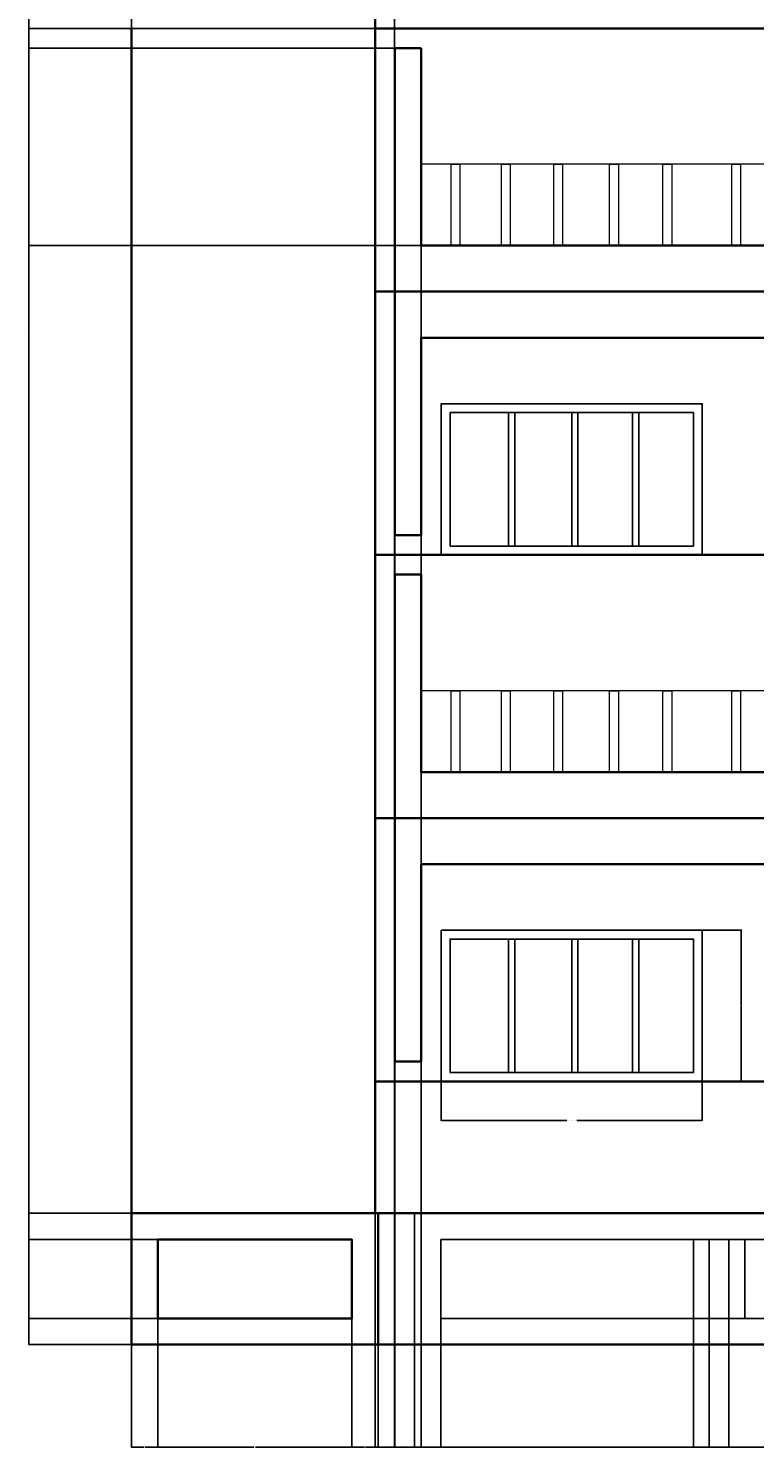
# Model space of a CAD drawing. Units: inches. Extents: x -26 to 668, y -42 to 976.
# Tile 1 of 3: x -26 to 305, y -42 to 605. Entities that reach past the tile are written whole.
import ezdxf

# ---------------------------------------------------------------- set-up
doc = ezdxf.new("R2010")
doc.units = ezdxf.units.IN
doc.header["$MEASUREMENT"] = 0
for name, color, linetype, lineweight in [('A-ANNO-DIMS', 2, 'Continuous', 18), ('A-DOOR', 3, 'Continuous', 25), ('A-ELEV', 7, 'Continuous', 35), ('A-FLOR-HRAL', 8, 'Continuous', 18), ('A-GLAZ', 4, 'Continuous', 25)]:
    doc.layers.add(name, color=color, linetype=linetype, lineweight=lineweight)
doc.styles.get("Standard").update_dxf_attribs({"font": 'arial.ttf'})
doc.dimstyles.get("Standard").update_dxf_attribs({"dimtxt": 0.18, "dimasz": 0.18, "dimexe": 0.18, "dimexo": 0.0625, "dimgap": 0.09, "dimtad": 0, "dimtih": 1, "dimtoh": 1, "dimdec": 4, "dimzin": 0, "dimdsep": 46, "dimtxsty": 'Standard', "dimcen": 0.09, "dimadec": 0, "dimazin": 0, "dimtfac": 1, "dimtdec": 4, "dimtofl": 0, "dimtmove": 0, "dimatfit": 3, "dimfxl": 1, "dimtolj": 1, "dimtzin": 0, "dimarcsym": 0})

# ---------------------------------------------------------------- blocks, each defined once
blk = doc.blocks.new('WIN-SLIDING-4P')
for p, q in [((192.66, 189.86), (192.66, 128.96)), ((195.46, 189.86), (195.46, 128.96)), ((221.46, 189.86), (221.46, 128.96)), ((224.25, 189.86), (224.25, 128.96)), ((249.2, 189.86), (249.2, 128.96)), ((251.99, 189.86), (251.99, 128.96))]:
    blk.add_line(p, q)
for points in [[(162.01, 124.96), (280.91, 124.96), (280.91, 193.86), (162.01, 193.86)], [(166.01, 128.96), (276.91, 128.96), (276.91, 189.86), (166.01, 189.86)]]:
    blk.add_lwpolyline(points, close=True)
blk = doc.blocks.new('RAILING-BALCONY')
for points in [[(331.17, 145.96), (599.79, 145.96), (599.79, 183.06), (331.17, 183.06)], [(344.86, 183.06), (348.85, 183.06), (348.85, 145.96), (344.86, 145.96)], [(367.74, 183.06), (371.72, 183.06), (371.72, 145.96), (367.74, 145.96)], [(391.66, 183.06), (395.64, 183.06), (395.64, 145.96), (391.66, 145.96)], [(417.04, 183.06), (421.03, 183.06), (421.03, 145.96), (417.04, 145.96)], [(441.38, 183.06), (445.37, 183.06), (445.37, 145.96), (441.38, 145.96)], [(472.69, 183.06), (476.68, 183.06), (476.68, 145.96), (472.69, 145.96)], [(501.02, 183.06), (505, 183.06), (505, 145.96), (501.02, 145.96)], [(530.39, 183.06), (534.38, 183.06), (534.38, 145.96), (530.39, 145.96)], [(556.62, 183.06), (560.61, 183.06), (560.61, 145.96), (556.62, 145.96)], [(580.54, 183.06), (584.53, 183.06), (584.53, 145.96), (580.54, 145.96)]]:
    blk.add_lwpolyline(points, close=True)
blk = doc.blocks.new('*D5')
at = {"layer": 'A-ANNO-DIMS', "color": 0, "lineweight": -2, "transparency": 16777216}
for p, q in [((162.01, 124.9), (162.01, 106.95)), ((280.91, 124.9), (280.91, 106.95)), ((162.19, 107.13), (219.17, 107.13)), ((280.73, 107.13), (223.74, 107.13))]:
    blk.add_line(p, q, dxfattribs=at)
at = {"layer": 'A-ANNO-DIMS', "color": 0, "transparency": 16777216}
for points in [[(162.19, 107.16), (162.19, 107.1), (162.01, 107.13)], [(280.73, 107.16), (280.73, 107.1), (280.91, 107.13)]]:
    blk.add_solid(points, dxfattribs=at)
at = {"layer": 'Defpoints', "color": 0, "transparency": 16777216}
for p in [(162.01, 124.96), (280.91, 124.96), (280.91, 107.13)]:
    blk.add_point(p, dxfattribs=at)
at = {"layer": 'A-ANNO-DIMS', "color": 0, "transparency": 16777216, "insert": (221.46, 107.13), "char_height": 0.18, "attachment_point": 5}
blk.add_mtext('\\A1;4-PANEL SLIDING WINDOW 119 TYP.', dxfattribs=at)
blk = doc.blocks.new('*D6')
at = {"layer": 'A-ANNO-DIMS', "color": 0, "lineweight": -2, "transparency": 16777216}
for p, q in [((280.97, 193.86), (298.92, 193.86)), ((298.74, 193.68), (298.74, 159.59)), ((298.74, 125.14), (298.74, 159.23)), ((280.97, 124.96), (298.92, 124.96))]:
    blk.add_line(p, q, dxfattribs=at)
at = {"layer": 'A-ANNO-DIMS', "color": 0, "transparency": 16777216}
for points in [[(298.71, 193.68), (298.77, 193.68), (298.74, 193.86)], [(298.71, 125.14), (298.77, 125.14), (298.74, 124.96)]]:
    blk.add_solid(points, dxfattribs=at)
at = {"layer": 'Defpoints', "color": 0, "transparency": 16777216}
for p in [(280.91, 193.86), (298.74, 193.86), (280.91, 124.96)]:
    blk.add_point(p, dxfattribs=at)
at = {"layer": 'A-ANNO-DIMS', "color": 0, "transparency": 16777216, "insert": (298.74, 159.41), "char_height": 0.18, "attachment_point": 5}
blk.add_mtext('\\A1;69 TYP.', dxfattribs=at)
blk = doc.blocks.new('*D8')
at = {"layer": 'A-ANNO-DIMS', "color": 0, "lineweight": -2, "transparency": 16777216}
for p, q in [((140.59, 928.96), (-26.14, 928.96)), ((-25.96, 928.78), (-25.96, 467.14)), ((-25.96, 5.14), (-25.96, 466.78)), ((20.73, 4.96), (-26.14, 4.96))]:
    blk.add_line(p, q, dxfattribs=at)
at = {"layer": 'A-ANNO-DIMS', "color": 0, "transparency": 16777216}
for points in [[(-25.99, 928.78), (-25.93, 928.78), (-25.96, 928.96)], [(-25.99, 5.14), (-25.93, 5.14), (-25.96, 4.96)]]:
    blk.add_solid(points, dxfattribs=at)
at = {"layer": 'Defpoints', "color": 0, "transparency": 16777216}
for p in [(-25.96, 928.96), (140.65, 928.96), (20.79, 4.96)]:
    blk.add_point(p, dxfattribs=at)
at = {"layer": 'A-ANNO-DIMS', "color": 0, "transparency": 16777216, "insert": (-25.96, 466.96), "char_height": 0.18, "attachment_point": 5}
blk.add_mtext('\\A1;924', dxfattribs=at)
blk = doc.blocks.new('*D22')
at = {"layer": 'A-ANNO-DIMS', "color": 0, "lineweight": -2, "transparency": 16777216}
for p, q in [((140.65, 844.9), (140.65, -41.97)), ((483.43, 844.9), (483.43, -41.97)), ((140.83, -41.79), (311.65, -41.79)), ((483.25, -41.79), (312.43, -41.79))]:
    blk.add_line(p, q, dxfattribs=at)
at = {"layer": 'A-ANNO-DIMS', "color": 0, "transparency": 16777216}
for points in [[(140.83, -41.76), (140.83, -41.82), (140.65, -41.79)], [(483.25, -41.76), (483.25, -41.82), (483.43, -41.79)]]:
    blk.add_solid(points, dxfattribs=at)
at = {"layer": 'Defpoints', "color": 0, "transparency": 16777216}
for p in [(140.65, 844.96), (483.43, 844.96), (483.43, -41.79)]:
    blk.add_point(p, dxfattribs=at)
at = {"layer": 'A-ANNO-DIMS', "color": 0, "transparency": 16777216, "insert": (312.04, -41.79), "char_height": 0.18, "attachment_point": 5}
blk.add_mtext('\\A1;342.8', dxfattribs=at)
blk = doc.blocks.new('*D28')
at = {"layer": 'A-ANNO-DIMS', "color": 0, "lineweight": -2, "transparency": 16777216}
for p, q in [((131.83, 604.9), (131.83, -41.97)), ((140.83, 595.9), (140.83, -41.97)), ((132.01, -41.79), (136.19, -41.79)), ((140.65, -41.79), (136.48, -41.79))]:
    blk.add_line(p, q, dxfattribs=at)
at = {"layer": 'A-ANNO-DIMS', "color": 0, "transparency": 16777216}
for points in [[(132.01, -41.76), (132.01, -41.82), (131.83, -41.79)], [(140.65, -41.76), (140.65, -41.82), (140.83, -41.79)]]:
    blk.add_solid(points, dxfattribs=at)
at = {"layer": 'Defpoints', "color": 0, "transparency": 16777216}
for p in [(131.83, 604.96), (140.83, 595.96), (140.83, -41.79)]:
    blk.add_point(p, dxfattribs=at)
at = {"layer": 'A-ANNO-DIMS', "color": 0, "transparency": 16777216, "insert": (136.33, -41.79), "char_height": 0.18, "attachment_point": 5}
blk.add_mtext('\\A1;9', dxfattribs=at)
blk = doc.blocks.new('*D29')
at = {"layer": 'A-ANNO-DIMS', "color": 0, "lineweight": -2, "transparency": 16777216}
for p, q in [((140.83, 595.9), (140.83, -41.97)), ((152.83, 505.9), (152.83, -41.97)), ((141.01, -41.79), (146.63, -41.79)), ((152.65, -41.79), (147.04, -41.79))]:
    blk.add_line(p, q, dxfattribs=at)
at = {"layer": 'A-ANNO-DIMS', "color": 0, "transparency": 16777216}
for points in [[(141.01, -41.76), (141.01, -41.82), (140.83, -41.79)], [(152.65, -41.76), (152.65, -41.82), (152.83, -41.79)]]:
    blk.add_solid(points, dxfattribs=at)
at = {"layer": 'Defpoints', "color": 0, "transparency": 16777216}
for p in [(140.83, 595.96), (152.83, 505.96), (152.83, -41.79)]:
    blk.add_point(p, dxfattribs=at)
at = {"layer": 'A-ANNO-DIMS', "color": 0, "transparency": 16777216, "insert": (146.83, -41.79), "char_height": 0.18, "attachment_point": 5}
blk.add_mtext('\\A1;12', dxfattribs=at)
blk = doc.blocks.new('*D30')
at = {"layer": 'A-ANNO-DIMS', "color": 0, "lineweight": -2, "transparency": 16777216}
for p, q in [((152.83, 505.9), (152.83, -41.97)), ((310.17, 505.9), (310.17, -41.97)), ((153.01, -41.79), (231.05, -41.79)), ((309.99, -41.79), (231.96, -41.79))]:
    blk.add_line(p, q, dxfattribs=at)
at = {"layer": 'A-ANNO-DIMS', "color": 0, "transparency": 16777216}
for points in [[(153.01, -41.76), (153.01, -41.82), (152.83, -41.79)], [(309.99, -41.76), (309.99, -41.82), (310.17, -41.79)]]:
    blk.add_solid(points, dxfattribs=at)
at = {"layer": 'Defpoints', "color": 0, "transparency": 16777216}
for p in [(152.83, 505.96), (310.17, 505.96), (310.17, -41.79)]:
    blk.add_point(p, dxfattribs=at)
at = {"layer": 'A-ANNO-DIMS', "color": 0, "transparency": 16777216, "insert": (231.5, -41.79), "char_height": 0.18, "attachment_point": 5}
blk.add_mtext('\\A1;157.34', dxfattribs=at)
blk = doc.blocks.new('*D38')
at = {"layer": 'A-ANNO-DIMS', "color": 0, "lineweight": -2, "transparency": 16777216}
for p, q in [((140.77, 595.96), (-26.14, 595.96)), ((-25.96, 595.78), (-25.96, 551.14)), ((-25.96, 506.14), (-25.96, 550.78)), ((152.77, 505.96), (-26.14, 505.96))]:
    blk.add_line(p, q, dxfattribs=at)
at = {"layer": 'A-ANNO-DIMS', "color": 0, "transparency": 16777216}
for points in [[(-25.99, 595.78), (-25.93, 595.78), (-25.96, 595.96)], [(-25.99, 506.14), (-25.93, 506.14), (-25.96, 505.96)]]:
    blk.add_solid(points, dxfattribs=at)
at = {"layer": 'Defpoints', "color": 0, "transparency": 16777216}
for p in [(-25.96, 595.96), (140.83, 595.96), (152.83, 505.96)]:
    blk.add_point(p, dxfattribs=at)
at = {"layer": 'A-ANNO-DIMS', "color": 0, "transparency": 16777216, "insert": (-25.96, 550.96), "char_height": 0.18, "attachment_point": 5}
blk.add_mtext('\\A1;90', dxfattribs=at)
blk = doc.blocks.new('*D39')
at = {"layer": 'A-ANNO-DIMS', "color": 0, "lineweight": -2, "transparency": 16777216}
for p, q in [((131.77, 604.96), (-26.14, 604.96)), ((-25.96, 604.78), (-25.96, 600.64)), ((140.77, 595.96), (-26.14, 595.96)), ((-25.96, 596.14), (-25.96, 600.28))]:
    blk.add_line(p, q, dxfattribs=at)
at = {"layer": 'A-ANNO-DIMS', "color": 0, "transparency": 16777216}
for points in [[(-25.99, 604.78), (-25.93, 604.78), (-25.96, 604.96)], [(-25.99, 596.14), (-25.93, 596.14), (-25.96, 595.96)]]:
    blk.add_solid(points, dxfattribs=at)
at = {"layer": 'Defpoints', "color": 0, "transparency": 16777216}
for p in [(-25.96, 604.96), (131.83, 604.96), (140.83, 595.96)]:
    blk.add_point(p, dxfattribs=at)
at = {"layer": 'A-ANNO-DIMS', "color": 0, "transparency": 16777216, "insert": (-25.96, 600.46), "char_height": 0.18, "attachment_point": 5}
blk.add_mtext('\\A1;9', dxfattribs=at)
blk = doc.blocks.new('*D40')
at = {"layer": 'A-ANNO-DIMS', "color": 0, "lineweight": -2, "transparency": 16777216}
for p, q in [((140.77, 613.96), (-26.14, 613.96)), ((-25.96, 613.78), (-25.96, 609.64)), ((-25.96, 605.14), (-25.96, 609.28)), ((131.77, 604.96), (-26.14, 604.96))]:
    blk.add_line(p, q, dxfattribs=at)
at = {"layer": 'A-ANNO-DIMS', "color": 0, "transparency": 16777216}
for points in [[(-25.99, 613.78), (-25.93, 613.78), (-25.96, 613.96)], [(-25.99, 605.14), (-25.93, 605.14), (-25.96, 604.96)]]:
    blk.add_solid(points, dxfattribs=at)
at = {"layer": 'Defpoints', "color": 0, "transparency": 16777216}
for p in [(-25.96, 613.96), (140.83, 613.96), (131.83, 604.96)]:
    blk.add_point(p, dxfattribs=at)
at = {"layer": 'A-ANNO-DIMS', "color": 0, "transparency": 16777216, "insert": (-25.96, 609.46), "char_height": 0.18, "attachment_point": 5}
blk.add_mtext('\\A1;9', dxfattribs=at)
blk = doc.blocks.new('*D47')
at = {"layer": 'A-ANNO-DIMS', "color": 0, "lineweight": -2, "transparency": 16777216}
for p, q in [((32.79, 16.9), (32.79, -41.97)), ((20.79, 4.9), (20.79, -41.97)), ((20.97, -41.79), (26.58, -41.79)), ((32.61, -41.79), (27, -41.79))]:
    blk.add_line(p, q, dxfattribs=at)
at = {"layer": 'A-ANNO-DIMS', "color": 0, "transparency": 16777216}
for points in [[(20.97, -41.76), (20.97, -41.82), (20.79, -41.79)], [(32.61, -41.76), (32.61, -41.82), (32.79, -41.79)]]:
    blk.add_solid(points, dxfattribs=at)
at = {"layer": 'Defpoints', "color": 0, "transparency": 16777216}
for p in [(32.79, 16.96), (20.79, 4.96), (32.79, -41.79)]:
    blk.add_point(p, dxfattribs=at)
at = {"layer": 'A-ANNO-DIMS', "color": 0, "transparency": 16777216, "insert": (26.79, -41.79), "char_height": 0.18, "attachment_point": 5}
blk.add_mtext('\\A1;12', dxfattribs=at)
blk = doc.blocks.new('*D48')
at = {"layer": 'A-ANNO-DIMS', "color": 0, "lineweight": -2, "transparency": 16777216}
for p, q in [((32.79, 16.9), (32.79, -41.97)), ((121.22, 16.9), (121.22, -41.97)), ((32.97, -41.79), (76.61, -41.79)), ((121.04, -41.79), (77.4, -41.79))]:
    blk.add_line(p, q, dxfattribs=at)
at = {"layer": 'A-ANNO-DIMS', "color": 0, "transparency": 16777216}
for points in [[(32.97, -41.76), (32.97, -41.82), (32.79, -41.79)], [(121.04, -41.76), (121.04, -41.82), (121.22, -41.79)]]:
    blk.add_solid(points, dxfattribs=at)
at = {"layer": 'Defpoints', "color": 0, "transparency": 16777216}
for p in [(32.79, 16.96), (121.22, 16.96), (121.22, -41.79)]:
    blk.add_point(p, dxfattribs=at)
at = {"layer": 'A-ANNO-DIMS', "color": 0, "transparency": 16777216, "insert": (77.01, -41.79), "char_height": 0.18, "attachment_point": 5}
blk.add_mtext('\\A1;88.43', dxfattribs=at)
blk = doc.blocks.new('*D49')
at = {"layer": 'A-ANNO-DIMS', "color": 0, "lineweight": -2, "transparency": 16777216}
for p, q in [((121.22, 16.9), (121.22, -41.97)), ((133.22, 4.9), (133.22, -41.97)), ((121.4, -41.79), (127.01, -41.79)), ((133.04, -41.79), (127.43, -41.79))]:
    blk.add_line(p, q, dxfattribs=at)
at = {"layer": 'A-ANNO-DIMS', "color": 0, "transparency": 16777216}
for points in [[(121.4, -41.76), (121.4, -41.82), (121.22, -41.79)], [(133.04, -41.76), (133.04, -41.82), (133.22, -41.79)]]:
    blk.add_solid(points, dxfattribs=at)
at = {"layer": 'Defpoints', "color": 0, "transparency": 16777216}
for p in [(121.22, 16.96), (133.22, 4.96), (133.22, -41.79)]:
    blk.add_point(p, dxfattribs=at)
at = {"layer": 'A-ANNO-DIMS', "color": 0, "transparency": 16777216, "insert": (127.22, -41.79), "char_height": 0.18, "attachment_point": 5}
blk.add_mtext('\\A1;12', dxfattribs=at)
blk = doc.blocks.new('*D50')
at = {"layer": 'A-ANNO-DIMS', "color": 0, "lineweight": -2, "transparency": 16777216}
for p, q in [((133.22, 4.9), (133.22, -41.97)), ((149.75, 4.9), (149.75, -41.97)), ((133.4, -41.79), (141.03, -41.79)), ((149.57, -41.79), (141.94, -41.79))]:
    blk.add_line(p, q, dxfattribs=at)
at = {"layer": 'A-ANNO-DIMS', "color": 0, "transparency": 16777216}
for points in [[(133.4, -41.76), (133.4, -41.82), (133.22, -41.79)], [(149.57, -41.76), (149.57, -41.82), (149.75, -41.79)]]:
    blk.add_solid(points, dxfattribs=at)
at = {"layer": 'Defpoints', "color": 0, "transparency": 16777216}
for p in [(133.22, 4.96), (149.75, 4.96), (149.75, -41.79)]:
    blk.add_point(p, dxfattribs=at)
at = {"layer": 'A-ANNO-DIMS', "color": 0, "transparency": 16777216, "insert": (141.49, -41.79), "char_height": 0.18, "attachment_point": 5}
blk.add_mtext('\\A1;16.527', dxfattribs=at)
blk = doc.blocks.new('*D51')
at = {"layer": 'A-ANNO-DIMS', "color": 0, "lineweight": -2, "transparency": 16777216}
for p, q in [((161.75, 16.9), (161.75, -41.97)), ((149.75, 4.9), (149.75, -41.97)), ((149.93, -41.79), (155.54, -41.79)), ((161.57, -41.79), (155.96, -41.79))]:
    blk.add_line(p, q, dxfattribs=at)
at = {"layer": 'A-ANNO-DIMS', "color": 0, "transparency": 16777216}
for points in [[(149.93, -41.76), (149.93, -41.82), (149.75, -41.79)], [(161.57, -41.76), (161.57, -41.82), (161.75, -41.79)]]:
    blk.add_solid(points, dxfattribs=at)
at = {"layer": 'Defpoints', "color": 0, "transparency": 16777216}
for p in [(161.75, 16.96), (149.75, 4.96), (161.75, -41.79)]:
    blk.add_point(p, dxfattribs=at)
at = {"layer": 'A-ANNO-DIMS', "color": 0, "transparency": 16777216, "insert": (155.75, -41.79), "char_height": 0.18, "attachment_point": 5}
blk.add_mtext('\\A1;12', dxfattribs=at)
blk = doc.blocks.new('*D52')
at = {"layer": 'A-ANNO-DIMS', "color": 0, "lineweight": -2, "transparency": 16777216}
for p, q in [((161.75, 16.9), (161.75, -41.97)), ((276.93, 16.9), (276.93, -41.97)), ((161.93, -41.79), (218.89, -41.79)), ((276.75, -41.79), (219.8, -41.79))]:
    blk.add_line(p, q, dxfattribs=at)
at = {"layer": 'A-ANNO-DIMS', "color": 0, "transparency": 16777216}
for points in [[(161.93, -41.76), (161.93, -41.82), (161.75, -41.79)], [(276.75, -41.76), (276.75, -41.82), (276.93, -41.79)]]:
    blk.add_solid(points, dxfattribs=at)
at = {"layer": 'Defpoints', "color": 0, "transparency": 16777216}
for p in [(161.75, 16.96), (276.93, 16.96), (276.93, -41.79)]:
    blk.add_point(p, dxfattribs=at)
at = {"layer": 'A-ANNO-DIMS', "color": 0, "transparency": 16777216, "insert": (219.34, -41.79), "char_height": 0.18, "attachment_point": 5}
blk.add_mtext('\\A1;115.18', dxfattribs=at)
blk = doc.blocks.new('*D53')
at = {"layer": 'A-ANNO-DIMS', "color": 0, "lineweight": -2, "transparency": 16777216}
for p, q in [((276.93, 16.9), (276.93, -41.97)), ((284.11, 16.9), (284.11, -41.97)), ((277.11, -41.79), (280.13, -41.79)), ((283.93, -41.79), (280.91, -41.79))]:
    blk.add_line(p, q, dxfattribs=at)
at = {"layer": 'A-ANNO-DIMS', "color": 0, "transparency": 16777216}
for points in [[(277.11, -41.76), (277.11, -41.82), (276.93, -41.79)], [(283.93, -41.76), (283.93, -41.82), (284.11, -41.79)]]:
    blk.add_solid(points, dxfattribs=at)
at = {"layer": 'Defpoints', "color": 0, "transparency": 16777216}
for p in [(276.93, 16.96), (284.11, 16.96), (284.11, -41.79)]:
    blk.add_point(p, dxfattribs=at)
at = {"layer": 'A-ANNO-DIMS', "color": 0, "transparency": 16777216, "insert": (280.52, -41.79), "char_height": 0.18, "attachment_point": 5}
blk.add_mtext('\\A1;7.177', dxfattribs=at)
blk = doc.blocks.new('*D54')
at = {"layer": 'A-ANNO-DIMS', "color": 0, "lineweight": -2, "transparency": 16777216}
for p, q in [((284.11, 16.9), (284.11, -41.97)), ((293.12, 16.9), (293.12, -41.97)), ((284.29, -41.79), (288.22, -41.79)), ((292.94, -41.79), (289.01, -41.79))]:
    blk.add_line(p, q, dxfattribs=at)
at = {"layer": 'A-ANNO-DIMS', "color": 0, "transparency": 16777216}
for points in [[(284.29, -41.76), (284.29, -41.82), (284.11, -41.79)], [(292.94, -41.76), (292.94, -41.82), (293.12, -41.79)]]:
    blk.add_solid(points, dxfattribs=at)
at = {"layer": 'Defpoints', "color": 0, "transparency": 16777216}
for p in [(284.11, 16.96), (293.12, 16.96), (293.12, -41.79)]:
    blk.add_point(p, dxfattribs=at)
at = {"layer": 'A-ANNO-DIMS', "color": 0, "transparency": 16777216, "insert": (288.61, -41.79), "char_height": 0.18, "attachment_point": 5}
blk.add_mtext('\\A1;9.007', dxfattribs=at)
blk = doc.blocks.new('*D55')
at = {"layer": 'A-ANNO-DIMS', "color": 0, "lineweight": -2, "transparency": 16777216}
for p, q in [((293.12, 16.9), (293.12, -41.97)), ((381.21, 16.9), (381.21, -41.97)), ((293.3, -41.79), (336.86, -41.79)), ((381.03, -41.79), (337.47, -41.79))]:
    blk.add_line(p, q, dxfattribs=at)
at = {"layer": 'A-ANNO-DIMS', "color": 0, "transparency": 16777216}
for points in [[(293.3, -41.76), (293.3, -41.82), (293.12, -41.79)], [(381.03, -41.76), (381.03, -41.82), (381.21, -41.79)]]:
    blk.add_solid(points, dxfattribs=at)
at = {"layer": 'Defpoints', "color": 0, "transparency": 16777216}
for p in [(293.12, 16.96), (381.21, 16.96), (381.21, -41.79)]:
    blk.add_point(p, dxfattribs=at)
at = {"layer": 'A-ANNO-DIMS', "color": 0, "transparency": 16777216, "insert": (337.16, -41.79), "char_height": 0.18, "attachment_point": 5}
blk.add_mtext('\\A1;88.1', dxfattribs=at)
blk = doc.blocks.new('*D59')
at = {"layer": 'A-ANNO-DIMS', "color": 0, "lineweight": -2, "transparency": 16777216}
for p, q in [((32.73, 16.96), (-26.14, 16.96)), ((-25.96, 16.78), (-25.96, 11.14)), ((-25.96, 5.14), (-25.96, 10.78)), ((20.73, 4.96), (-26.14, 4.96))]:
    blk.add_line(p, q, dxfattribs=at)
at = {"layer": 'A-ANNO-DIMS', "color": 0, "transparency": 16777216}
for points in [[(-25.99, 16.78), (-25.93, 16.78), (-25.96, 16.96)], [(-25.99, 5.14), (-25.93, 5.14), (-25.96, 4.96)]]:
    blk.add_solid(points, dxfattribs=at)
at = {"layer": 'Defpoints', "color": 0, "transparency": 16777216}
for p in [(-25.96, 16.96), (32.79, 16.96), (20.79, 4.96)]:
    blk.add_point(p, dxfattribs=at)
at = {"layer": 'A-ANNO-DIMS', "color": 0, "transparency": 16777216, "insert": (-25.96, 10.96), "char_height": 0.18, "attachment_point": 5}
blk.add_mtext('\\A1;12', dxfattribs=at)
blk = doc.blocks.new('*D60')
at = {"layer": 'A-ANNO-DIMS', "color": 0, "lineweight": -2, "transparency": 16777216}
for p, q in [((32.73, 52.96), (-26.14, 52.96)), ((-25.96, 52.78), (-25.96, 35.14)), ((-25.96, 17.14), (-25.96, 34.78)), ((32.73, 16.96), (-26.14, 16.96))]:
    blk.add_line(p, q, dxfattribs=at)
at = {"layer": 'A-ANNO-DIMS', "color": 0, "transparency": 16777216}
for points in [[(-25.99, 52.78), (-25.93, 52.78), (-25.96, 52.96)], [(-25.99, 17.14), (-25.93, 17.14), (-25.96, 16.96)]]:
    blk.add_solid(points, dxfattribs=at)
at = {"layer": 'Defpoints', "color": 0, "transparency": 16777216}
for p in [(-25.96, 52.96), (32.79, 52.96), (32.79, 16.96)]:
    blk.add_point(p, dxfattribs=at)
at = {"layer": 'A-ANNO-DIMS', "color": 0, "transparency": 16777216, "insert": (-25.96, 34.96), "char_height": 0.18, "attachment_point": 5}
blk.add_mtext('\\A1;36', dxfattribs=at)
blk = doc.blocks.new('*D61')
at = {"layer": 'A-ANNO-DIMS', "color": 0, "lineweight": -2, "transparency": 16777216}
for p, q in [((20.73, 64.96), (-26.14, 64.96)), ((-25.96, 64.78), (-25.96, 59.14)), ((-25.96, 53.14), (-25.96, 58.78)), ((32.73, 52.96), (-26.14, 52.96))]:
    blk.add_line(p, q, dxfattribs=at)
at = {"layer": 'A-ANNO-DIMS', "color": 0, "transparency": 16777216}
for points in [[(-25.99, 64.78), (-25.93, 64.78), (-25.96, 64.96)], [(-25.99, 53.14), (-25.93, 53.14), (-25.96, 52.96)]]:
    blk.add_solid(points, dxfattribs=at)
at = {"layer": 'Defpoints', "color": 0, "transparency": 16777216}
for p in [(-25.96, 64.96), (20.79, 64.96), (32.79, 52.96)]:
    blk.add_point(p, dxfattribs=at)
at = {"layer": 'A-ANNO-DIMS', "color": 0, "transparency": 16777216, "insert": (-25.96, 58.96), "char_height": 0.18, "attachment_point": 5}
blk.add_mtext('\\A1;12', dxfattribs=at)
blk = doc.blocks.new('*D65')
at = {"layer": 'A-ANNO-DIMS', "color": 0, "lineweight": -2, "transparency": 16777216}
for p, q in [((20.79, 65.02), (20.79, 975.89)), ((20.97, 975.71), (75.86, 975.71)), ((131.65, 975.71), (76.77, 975.71)), ((131.83, 65.02), (131.83, 975.89))]:
    blk.add_line(p, q, dxfattribs=at)
at = {"layer": 'A-ANNO-DIMS', "color": 0, "transparency": 16777216}
for points in [[(20.97, 975.74), (20.97, 975.68), (20.79, 975.71)], [(131.65, 975.74), (131.65, 975.68), (131.83, 975.71)]]:
    blk.add_solid(points, dxfattribs=at)
at = {"layer": 'Defpoints', "color": 0, "transparency": 16777216}
for p in [(131.83, 975.71), (20.79, 64.96), (131.83, 64.96)]:
    blk.add_point(p, dxfattribs=at)
at = {"layer": 'A-ANNO-DIMS', "color": 0, "transparency": 16777216, "insert": (76.31, 975.71), "char_height": 0.18, "attachment_point": 5}
blk.add_mtext('\\A1;111.04', dxfattribs=at)

msp = doc.modelspace()

# ---------------------------------------------------------------- linework, layer by layer
at = {"layer": 'A-DOOR'}
for points in [[(149.7506, 64.9609), (402.2206, 64.9609), (402.2206, 4.9609), (149.7506, 4.9609)], [(161.7506, 52.9609), (390.2206, 52.9609), (390.2206, 16.9609), (161.7506, 16.9609)], [(284.1079, 16.9609), (276.9308, 16.9609), (276.9308, 52.9609), (284.1079, 52.9609)], [(300.2922, 16.9609), (293.1151, 16.9609), (293.1151, 52.9609), (300.2922, 52.9609)]]:
    msp.add_lwpolyline(points, close=True, dxfattribs=at)
at = {"layer": 'A-ELEV'}
for p, q in [((131.8349, 844.9609), (131.8349, 64.9609)), ((140.8349, 484.9609), (140.8349, 595.9609)), ((140.8349, 595.9609), (152.8349, 595.9609)), ((140.8349, 244.9609), (140.8349, 355.9609)), ((140.8349, 355.9609), (152.8349, 355.9609)), ((140.8349, 244.9609), (140.8349, 133.9609)), ((140.8349, 133.9609), (152.8349, 133.9609)), ((20.7944, 124.9609), (20.7944, 4.9609)), ((620.7944, 124.9609), (131.8349, 124.9609)), ((20.7944, 64.9609), (620.7944, 64.9609)), ((20.7944, 4.9609), (620.7944, 4.9609))]:
    msp.add_line(p, q, dxfattribs=at)
for points in [[(20.7944, 604.9609), (20.7944, 484.9609)], [(131.8349, 484.9609), (620.7944, 484.9609), (620.7944, 604.9609), (131.8349, 604.9609)], [(331.1714, 505.9609), (152.8349, 505.9609), (152.8349, 595.9609)], [(20.7944, 484.9609), (20.7944, 364.9609)], [(131.8349, 364.9609), (620.7944, 364.9609), (620.7944, 484.9609), (131.8349, 484.9609)], [(140.8349, 484.9609), (140.8349, 373.9609), (152.8349, 373.9609)], [(331.1714, 463.9609), (152.8349, 463.9609), (152.8349, 373.9609)], [(20.7944, 364.9609), (20.7944, 244.9609)], [(131.8349, 244.9609), (620.7944, 244.9609), (620.7944, 364.9609), (131.8349, 364.9609)], [(131.8349, 244.9609), (131.8349, 364.9609), (504.2381, 364.9609)], [(331.1714, 265.9609), (152.8349, 265.9609), (152.8349, 355.9609)], [(20.7944, 244.9609), (20.7944, 124.9609)], [(131.8349, 124.9609), (620.7944, 124.9609), (620.7944, 244.9609), (131.8349, 244.9609)], [(504.2381, 124.9609), (131.8349, 124.9609), (131.8349, 244.9609), (504.2381, 244.9609)], [(488.5079, 244.9609), (131.8349, 244.9609), (131.8349, 124.9609), (488.5079, 124.9609)], [(331.1714, 223.9609), (152.8349, 223.9609), (152.8349, 133.9609)]]:
    msp.add_lwpolyline(points, dxfattribs=at)
for points in [[(20.7944, 64.9609), (133.2232, 64.9609), (133.2232, 4.9609), (20.7944, 4.9609)], [(32.7944, 52.9609), (121.2232, 52.9609), (121.2232, 16.9609), (32.7944, 16.9609)]]:
    msp.add_lwpolyline(points, close=True, dxfattribs=at)

# ---------------------------------------------------------------- block references
at = {"layer": 'A-FLOR-HRAL'}
for p in [(-178.3365, 360), (-178.3365, 120)]:
    msp.add_blockref('RAILING-BALCONY', p, dxfattribs=at)
at = {"layer": 'A-GLAZ'}
for p in [(0, 240), (0, 0)]:
    msp.add_blockref('WIN-SLIDING-4P', p, dxfattribs=at)

# ---------------------------------------------------------------- dimensions: what is measured, and where the dimension line sits
at = {"layer": 'A-ANNO-DIMS'}
for base, p1, p2, override, picture, middle in [((131.8349, 975.7109), (20.7944, 64.9609), (131.8349, 64.9609), {"dimdec": 2, "dimlfac": 1, "dimrnd": 0, "dimzin": 0, "dimdsep": 46, "dimlunit": 2}, '*D65', (76.3146, 975.7109)), ((483.4325, -41.7891), (140.6477, 844.9609), (483.4325, 844.9609), {"dimdec": 1, "dimlfac": 1, "dimrnd": 0, "dimzin": 0, "dimdsep": 46, "dimlunit": 2}, '*D22', (312.0401, -41.7891)), ((140.8349, -41.7891), (131.8349, 604.9609), (140.8349, 595.9609), {"dimdec": 0, "dimlfac": 1, "dimrnd": 0, "dimzin": 0, "dimdsep": 46, "dimlunit": 2}, '*D28', (136.3349, -41.7891)), ((152.8349, -41.7891), (140.8349, 595.9609), (152.8349, 505.9609), {"dimdec": 0, "dimlfac": 1, "dimrnd": 0, "dimzin": 0, "dimdsep": 46, "dimlunit": 2}, '*D29', (146.8349, -41.7891)), ((310.1714, -41.7891), (152.8349, 505.9609), (310.1714, 505.9609), {"dimdec": 2, "dimlfac": 1, "dimrnd": 0, "dimzin": 0, "dimdsep": 46, "dimlunit": 2}, '*D30', (231.5031, -41.7891)), ((32.7944, -41.7891), (20.7944, 4.9609), (32.7944, 16.9609), {"dimdec": 0, "dimlfac": 1, "dimrnd": 0, "dimzin": 0, "dimdsep": 46, "dimlunit": 2}, '*D47', (26.7944, -41.7891)), ((121.2232, -41.7891), (32.7944, 16.9609), (121.2232, 16.9609), {"dimdec": 2, "dimlfac": 1, "dimrnd": 0, "dimzin": 0, "dimdsep": 46, "dimlunit": 2}, '*D48', (77.0088, -41.7891)), ((133.2232, -41.7891), (121.2232, 16.9609), (133.2232, 4.9609), {"dimdec": 0, "dimlfac": 1, "dimrnd": 0, "dimzin": 0, "dimdsep": 46, "dimlunit": 2}, '*D49', (127.2232, -41.7891)), ((161.7506, -41.7891), (149.7506, 4.9609), (161.7506, 16.9609), {"dimdec": 0, "dimlfac": 1, "dimrnd": 0, "dimzin": 0, "dimdsep": 46, "dimlunit": 2}, '*D51', (155.7506, -41.7891)), ((276.9308, -41.7891), (161.7506, 16.9609), (276.9308, 16.9609), {"dimdec": 2, "dimlfac": 1, "dimrnd": 0, "dimzin": 0, "dimdsep": 46, "dimlunit": 2}, '*D52', (219.3407, -41.7891)), ((284.1079, -41.7891), (276.9308, 16.9609), (284.1079, 16.9609), {"dimdec": 3, "dimlfac": 1, "dimrnd": 0, "dimzin": 0, "dimdsep": 46, "dimlunit": 2}, '*D53', (280.5194, -41.7891)), ((293.1151, -41.7891), (284.1079, 16.9609), (293.1151, 16.9609), {"dimdec": 3, "dimlfac": 1, "dimrnd": 0, "dimzin": 0, "dimdsep": 46, "dimlunit": 2}, '*D54', (288.6115, -41.7891)), ((381.2134, -41.7891), (293.1151, 16.9609), (381.2134, 16.9609), {"dimdec": 1, "dimlfac": 1, "dimrnd": 0, "dimzin": 0, "dimdsep": 46, "dimlunit": 2}, '*D55', (337.1643, -41.7891)), ((149.7506, -41.7891), (133.2232, 4.9609), (149.7506, 4.9609), {"dimdec": 3, "dimlfac": 1, "dimrnd": 0, "dimzin": 0, "dimdsep": 46, "dimlunit": 2}, '*D50', (141.4869, -41.7891))]:
    dim = msp.add_linear_dim(base=base, p1=p1, p2=p2, dimstyle='Standard', override=override, dxfattribs=at)
    dim.commit()
    dim.dimension.update_dxf_attribs({"geometry": picture, "text_midpoint": middle})
for base, p1, p2, picture, middle in [((-25.9556, 928.9609), (20.7944, 4.9609), (140.6477, 928.9609), '*D8', (-25.9556, 466.9609)), ((-25.9556, 613.9609), (131.8349, 604.9609), (140.8349, 613.9609), '*D40', (-25.9556, 609.4609)), ((-25.9556, 604.9609), (140.8349, 595.9609), (131.8349, 604.9609), '*D39', (-25.9556, 600.4609)), ((-25.9556, 595.9609), (152.8349, 505.9609), (140.8349, 595.9609), '*D38', (-25.9556, 550.9609)), ((-25.9556, 64.9609), (32.7944, 52.9609), (20.7944, 64.9609), '*D61', (-25.9556, 58.9609)), ((-25.9556, 52.9609), (32.7944, 16.9609), (32.7944, 52.9609), '*D60', (-25.9556, 34.9609)), ((-25.9556, 16.9609), (20.7944, 4.9609), (32.7944, 16.9609), '*D59', (-25.9556, 10.9609))]:
    dim = msp.add_linear_dim(base=base, p1=p1, p2=p2, angle=90, dimstyle='Standard', override={"dimdec": 0, "dimlfac": 1, "dimrnd": 0, "dimzin": 0, "dimdsep": 46, "dimlunit": 2}, dxfattribs=at)
    dim.commit()
    dim.dimension.update_dxf_attribs({"geometry": picture, "text_midpoint": middle})
dim = msp.add_linear_dim(base=(298.7412, 193.8637), p1=(280.9068, 124.9609), p2=(280.9068, 193.8637), angle=90, text='<> TYP.', dimstyle='Standard', override={"dimdec": 0, "dimlfac": 1, "dimrnd": 0, "dimzin": 0, "dimdsep": 46, "dimlunit": 2}, dxfattribs=at)
dim.commit()
dim.dimension.update_dxf_attribs({"geometry": '*D6', "text_midpoint": (298.7412, 159.4123)})
dim = msp.add_linear_dim(base=(280.9068, 107.1265), p1=(162.0107, 124.9609), p2=(280.9068, 124.9609), text='4-PANEL SLIDING WINDOW <> TYP.', dimstyle='Standard', override={"dimdec": 0, "dimlfac": 1, "dimrnd": 0, "dimzin": 0, "dimdsep": 46, "dimlunit": 2}, dxfattribs=at)
dim.commit()
dim.dimension.update_dxf_attribs({"geometry": '*D5', "text_midpoint": (221.4587, 107.1265)})

doc.saveas('drawing.dxf')
